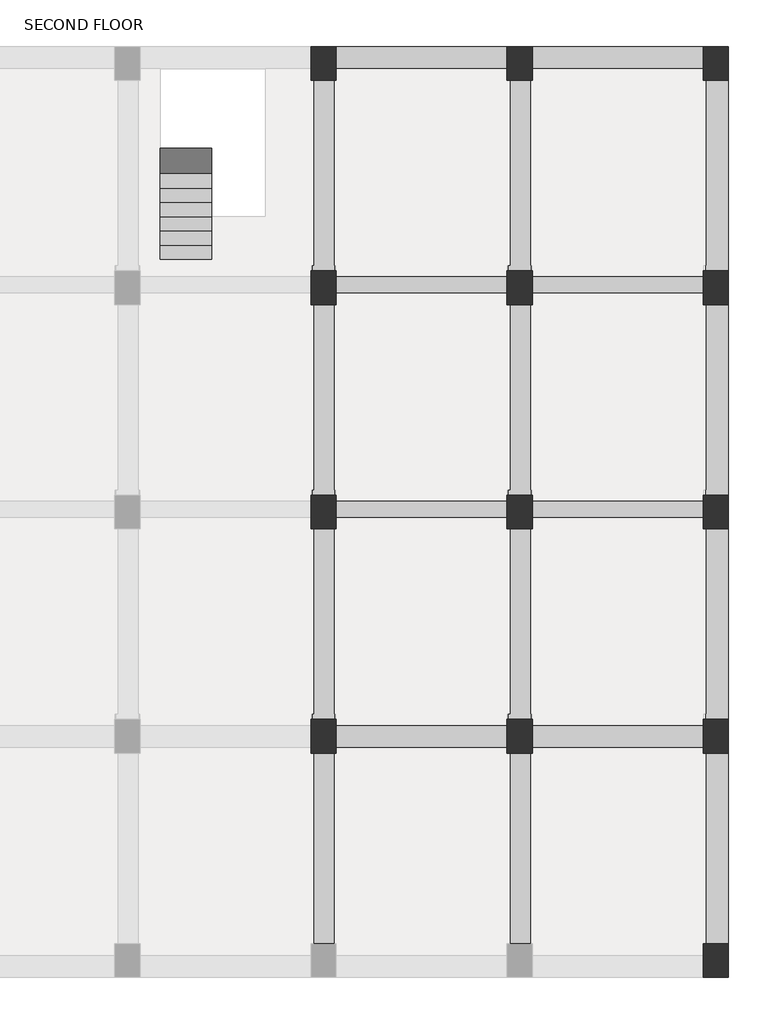
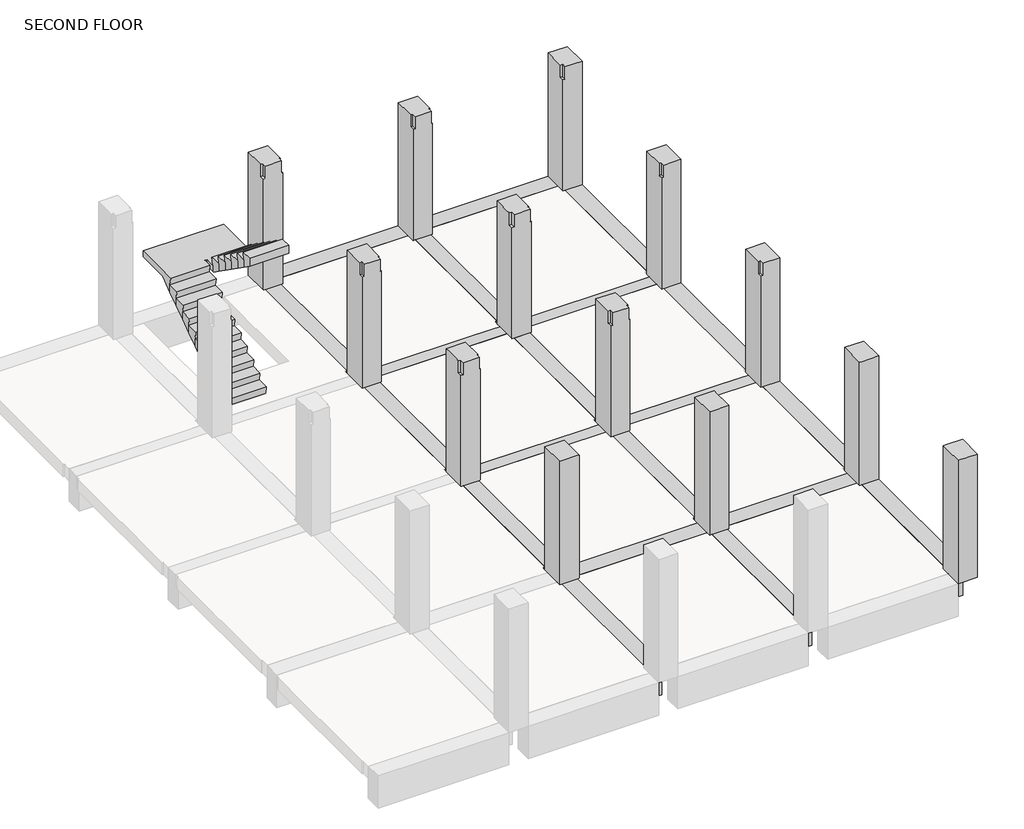
# One storey, part 3 of 3: 20 beams, 13 columns, 1 stair flight.
"""IFC4 building model written with IfcOpenShell, lengths in millimetres."""

from ifc_helpers import new_model, si_unit, origin, place, context, project, spatial, faceted_brep, element, save

model = new_model("IFC4")

# Units and contexts
model_context = context("Model", 3, world=origin())
ifc_project = project(units=[si_unit("LENGTHUNIT", "METRE", prefix="MILLI")], contexts=[model_context])

# Site, building, storey
site = spatial("IfcSite", under=ifc_project)
building = spatial("IfcBuilding", under=site)
storey = spatial("IfcBuildingStorey", under=building, Name="SECOND FLOOR", Elevation=6096.0)

# Beams
placement = place(None, origin())
element("IfcBeam", 1, ObjectType="M_Concrete-Rectangular Beam : 400 x 800mm", at=placement, inside=storey, context=model_context, shape_type="Brep", body=[
    faceted_brep([(7955.1115906, 15703.1212443, 6096.0), (8355.1115906, 15703.1212443, 6096.0), (8355.1115906, 19103.1212443, 6096.0), (7955.1115906, 19103.1212443, 6096.0), (7955.1115906, 15803.1212443, 6096.0), (7955.1115906, 15703.1212443, 5296.0), (7955.1115906, 19103.1212443, 5296.0), (8355.1115906, 15703.1212443, 5296.0), (8355.1115906, 19103.1212443, 5296.0)], [[[0, 1, 2, 3, 4]], [[5, 0, 4, 3, 6]], [[7, 5, 6, 8]], [[1, 7, 8, 2]], [[2, 8, 6, 3]], [[1, 0, 5, 7]]]),
])
element("IfcBeam", 2, ObjectType="M_Concrete-Rectangular Beam : 400 x 800mm", at=placement, inside=storey, context=model_context, shape_type="Brep", body=[
    faceted_brep([(7955.1115906, 11703.1212443, 6096.0), (8355.1115906, 11703.1212443, 6096.0), (8355.1115906, 15103.1212443, 6096.0), (7955.1115906, 15103.1212443, 6096.0), (7955.1115906, 11803.1212443, 6096.0), (7955.1115906, 11703.1212443, 5296.0), (7955.1115906, 15103.1212443, 5296.0), (8355.1115906, 11703.1212443, 5296.0), (8355.1115906, 15103.1212443, 5296.0)], [[[0, 1, 2, 3, 4]], [[5, 0, 4, 3, 6]], [[7, 5, 6, 8]], [[1, 7, 8, 2]], [[2, 8, 6, 3]], [[1, 0, 5, 7]]]),
])
element("IfcBeam", 3, ObjectType="M_Concrete-Rectangular Beam : 400 x 800mm", at=placement, inside=storey, context=model_context, shape_type="Brep", body=[
    faceted_brep([(7955.1115906, 7703.1212443, 6096.0), (8355.1115906, 7703.1212443, 6096.0), (8355.1115906, 11103.1212443, 6096.0), (7955.1115906, 11103.1212443, 6096.0), (7955.1115906, 7803.1212443, 6096.0), (7955.1115906, 7703.1212443, 5296.0), (7955.1115906, 11103.1212443, 5296.0), (8355.1115906, 7703.1212443, 5296.0), (8355.1115906, 11103.1212443, 5296.0)], [[[0, 1, 2, 3, 4]], [[5, 0, 4, 3, 6]], [[7, 5, 6, 8]], [[1, 7, 8, 2]], [[1, 0, 5, 7]], [[3, 2, 8, 6]]]),
])
element("IfcBeam", 4, ObjectType="M_Concrete-Rectangular Beam : 400 x 800mm", at=placement, inside=storey, context=model_context, shape_type="Brep", body=[
    faceted_brep([(8355.1115906, 7103.1212443, 6096.0), (7955.1115906, 7103.1212443, 6096.0), (7955.1115906, 3703.1212443, 6096.0), (8355.1115906, 3703.1212443, 6096.0), (7955.1115906, 7103.1212443, 5796.0), (7955.1115906, 7103.1212443, 5296.0), (7955.1115906, 3703.1212443, 5296.0), (7955.1115906, 3703.1212443, 5796.0), (8355.1115906, 7103.1212443, 5296.0), (8355.1115906, 3703.1212443, 5296.0)], [[[0, 1, 2, 3]], [[1, 4, 5, 6, 7, 2]], [[5, 8, 9, 6]], [[8, 0, 3, 9]], [[0, 8, 5, 4, 1]], [[3, 2, 7, 6, 9]]]),
])
element("IfcBeam", 5, ObjectType="M_Concrete-Rectangular Beam : 400 x 800mm", at=placement, inside=storey, context=model_context, shape_type="Brep", body=[
    faceted_brep([(1355.1115906, 19703.1212443, 6096.0), (1355.1115906, 19303.1212443, 6096.0), (4405.1115906, 19303.1212443, 6096.0), (4405.1115906, 19703.1212443, 6096.0), (1355.1115906, 19303.1212443, 5796.0), (1355.1115906, 19303.1212443, 5296.0), (4405.1115906, 19303.1212443, 5296.0), (4405.1115906, 19303.1212443, 5796.0), (1355.1115906, 19703.1212443, 5296.0), (4405.1115906, 19703.1212443, 5296.0)], [[[0, 1, 2, 3]], [[1, 4, 5, 6, 7, 2]], [[5, 8, 9, 6]], [[8, 0, 3, 9]], [[1, 0, 8, 5, 4]], [[3, 2, 7, 6, 9]]]),
])
element("IfcBeam", 6, ObjectType="M_Concrete-Rectangular Beam : 400 x 800mm", at=placement, inside=storey, context=model_context, shape_type="Brep", body=[
    faceted_brep([(4855.1115906, 19703.1212443, 6096.0), (4855.1115906, 19303.1212443, 6096.0), (7905.1115906, 19303.1212443, 6096.0), (7905.1115906, 19703.1212443, 6096.0), (4855.1115906, 19303.1212443, 5796.0), (4855.1115906, 19303.1212443, 5296.0), (7905.1115906, 19303.1212443, 5296.0), (7905.1115906, 19303.1212443, 5796.0), (4855.1115906, 19703.1212443, 5296.0), (7905.1115906, 19703.1212443, 5296.0)], [[[0, 1, 2, 3]], [[1, 4, 5, 6, 7, 2]], [[5, 8, 9, 6]], [[8, 0, 3, 9]], [[1, 0, 8, 5, 4]], [[3, 2, 7, 6, 9]]]),
])
element("IfcBeam", 7, ObjectType="M_Concrete-Rectangular Beam : 400 x 800mm", at=placement, inside=storey, context=model_context, shape_type="Brep", body=[
    faceted_brep([(1330.1115906, 15703.1212443, 6096.0), (1330.1115906, 15803.1212443, 6096.0), (1330.1115906, 19103.1212443, 6096.0), (955.1115906, 19103.1212443, 6096.0), (955.1115906, 15803.1212443, 6096.0), (930.1115906, 15803.1212443, 6096.0), (930.1115906, 15703.1212443, 6096.0), (930.1115906, 19103.1212443, 5296.0), (930.1115906, 15703.1212443, 5296.0), (930.1115906, 15803.1212443, 5796.0), (930.1115906, 19103.1212443, 5796.0), (1330.1115906, 19103.1212443, 5296.0), (1330.1115906, 15703.1212443, 5296.0), (955.1115906, 19103.1212443, 5796.0), (955.1115906, 15803.1212443, 5796.0)], [[[0, 1, 2, 3, 4, 5, 6]], [[7, 8, 6, 5, 9, 10]], [[7, 11, 12, 8]], [[11, 2, 1, 0, 12]], [[2, 11, 7, 10, 13, 3]], [[0, 6, 8, 12]], [[9, 14, 13, 10]], [[14, 4, 3, 13]], [[4, 14, 9, 5]]]),
])
element("IfcBeam", 8, ObjectType="M_Concrete-Rectangular Beam : 400 x 800mm", at=placement, inside=storey, context=model_context, shape_type="Brep", body=[
    faceted_brep([(1330.1115906, 11703.1212443, 6096.0), (1330.1115906, 11803.1212443, 6096.0), (1330.1115906, 15103.1212443, 6096.0), (955.1115906, 15103.1212443, 6096.0), (955.1115906, 11803.1212443, 6096.0), (930.1115906, 11803.1212443, 6096.0), (930.1115906, 11703.1212443, 6096.0), (930.1115906, 15103.1212443, 5296.0), (930.1115906, 11703.1212443, 5296.0), (930.1115906, 11803.1212443, 5796.0), (930.1115906, 15103.1212443, 5796.0), (1330.1115906, 15103.1212443, 5296.0), (1330.1115906, 11703.1212443, 5296.0), (955.1115906, 15103.1212443, 5796.0), (955.1115906, 11803.1212443, 5796.0)], [[[0, 1, 2, 3, 4, 5, 6]], [[7, 8, 6, 5, 9, 10]], [[8, 7, 11, 12]], [[2, 1, 0, 12, 11]], [[2, 11, 7, 10, 13, 3]], [[0, 6, 8, 12]], [[9, 14, 13, 10]], [[14, 4, 3, 13]], [[4, 14, 9, 5]]]),
])
element("IfcBeam", 9, ObjectType="M_Concrete-Rectangular Beam : 400 x 800mm", at=placement, inside=storey, context=model_context, shape_type="Brep", body=[
    faceted_brep([(1330.1115906, 7703.1212443, 6096.0), (1330.1115906, 7803.1212443, 6096.0), (1330.1115906, 11103.1212443, 6096.0), (955.1115906, 11103.1212443, 6096.0), (955.1115906, 7803.1212443, 6096.0), (930.1115906, 7803.1212443, 6096.0), (930.1115906, 7703.1212443, 6096.0), (930.1115906, 11103.1212443, 5296.0), (930.1115906, 7703.1212443, 5296.0), (930.1115906, 7803.1212443, 5796.0), (930.1115906, 11103.1212443, 5796.0), (1330.1115906, 11103.1212443, 5296.0), (1330.1115906, 7703.1212443, 5296.0), (955.1115906, 11103.1212443, 5796.0), (955.1115906, 7803.1212443, 5796.0)], [[[0, 1, 2, 3, 4, 5, 6]], [[7, 8, 6, 5, 9, 10]], [[7, 11, 12, 8]], [[11, 2, 1, 0, 12]], [[2, 11, 7, 10, 13, 3]], [[0, 6, 8, 12]], [[9, 14, 13, 10]], [[14, 4, 3, 13]], [[4, 14, 9, 5]]]),
])
element("IfcBeam", 10, ObjectType="M_Concrete-Rectangular Beam : 400 x 800mm", at=placement, inside=storey, context=model_context, shape_type="Brep", body=[
    faceted_brep([(1330.1115906, 3703.1212443, 6096.0), (1330.1115906, 7103.1212443, 6096.0), (955.1115906, 7103.1212443, 6096.0), (955.1115906, 3703.1212443, 6096.0), (930.1115906, 7103.1212443, 5296.0), (930.1115906, 3703.1212443, 5296.0), (930.1115906, 3703.1212443, 5796.0), (930.1115906, 7103.1212443, 5796.0), (1330.1115906, 7103.1212443, 5296.0), (1330.1115906, 3703.1212443, 5296.0), (1330.1115906, 7103.1212443, 5796.0), (1330.1115906, 3703.1212443, 5796.0), (955.1115906, 7103.1212443, 5796.0), (955.1115906, 3703.1212443, 5796.0)], [[[0, 1, 2, 3]], [[4, 5, 6, 7]], [[4, 8, 9, 5]], [[8, 10, 1, 0, 11, 9]], [[8, 4, 7, 12, 2, 1, 10]], [[5, 9, 11, 0, 3, 13, 6]], [[13, 12, 7, 6]], [[12, 13, 3, 2]]]),
])
element("IfcBeam", 11, ObjectType="M_Concrete-Rectangular Beam : 400 x 800mm", at=placement, inside=storey, context=model_context, shape_type="Brep", body=[
    faceted_brep([(4830.1115906, 15703.1212443, 6096.0), (4830.1115906, 15803.1212443, 6096.0), (4830.1115906, 19103.1212443, 6096.0), (4455.1115906, 19103.1212443, 6096.0), (4455.1115906, 15803.1212443, 6096.0), (4430.1115906, 15803.1212443, 6096.0), (4430.1115906, 15703.1212443, 6096.0), (4430.1115906, 19103.1212443, 5296.0), (4430.1115906, 15703.1212443, 5296.0), (4430.1115906, 15803.1212443, 5796.0), (4430.1115906, 19103.1212443, 5796.0), (4830.1115906, 19103.1212443, 5296.0), (4830.1115906, 15703.1212443, 5296.0), (4455.1115906, 19103.1212443, 5796.0), (4455.1115906, 15803.1212443, 5796.0)], [[[0, 1, 2, 3, 4, 5, 6]], [[7, 8, 6, 5, 9, 10]], [[8, 7, 11, 12]], [[2, 1, 0, 12, 11]], [[2, 11, 7, 10, 13, 3]], [[0, 6, 8, 12]], [[9, 14, 13, 10]], [[14, 4, 3, 13]], [[4, 14, 9, 5]]]),
])
element("IfcBeam", 12, ObjectType="M_Concrete-Rectangular Beam : 400 x 800mm", at=placement, inside=storey, context=model_context, shape_type="Brep", body=[
    faceted_brep([(4830.1115906, 11703.1212443, 6096.0), (4830.1115906, 11803.1212443, 6096.0), (4830.1115906, 15103.1212443, 6096.0), (4455.1115906, 15103.1212443, 6096.0), (4455.1115906, 11803.1212443, 6096.0), (4430.1115906, 11803.1212443, 6096.0), (4430.1115906, 11703.1212443, 6096.0), (4430.1115906, 15103.1212443, 5296.0), (4430.1115906, 11703.1212443, 5296.0), (4430.1115906, 11803.1212443, 5796.0), (4430.1115906, 15103.1212443, 5796.0), (4830.1115906, 15103.1212443, 5296.0), (4830.1115906, 11703.1212443, 5296.0), (4455.1115906, 15103.1212443, 5796.0), (4455.1115906, 11803.1212443, 5796.0)], [[[0, 1, 2, 3, 4, 5, 6]], [[7, 8, 6, 5, 9, 10]], [[7, 11, 12, 8]], [[11, 2, 1, 0, 12]], [[2, 11, 7, 10, 13, 3]], [[0, 6, 8, 12]], [[9, 14, 13, 10]], [[14, 4, 3, 13]], [[4, 14, 9, 5]]]),
])
element("IfcBeam", 13, ObjectType="M_Concrete-Rectangular Beam : 400 x 800mm", at=placement, inside=storey, context=model_context, shape_type="Brep", body=[
    faceted_brep([(4430.1115906, 7703.1212443, 6096.0), (4830.1115906, 7703.1212443, 6096.0), (4830.1115906, 7803.1212443, 6096.0), (4830.1115906, 11103.1212443, 6096.0), (4455.1115906, 11103.1212443, 6096.0), (4455.1115906, 7803.1212443, 6096.0), (4430.1115906, 7803.1212443, 6096.0), (4430.1115906, 7703.1212443, 5296.0), (4430.1115906, 7803.1212443, 5796.0), (4430.1115906, 11103.1212443, 5796.0), (4430.1115906, 11103.1212443, 5296.0), (4830.1115906, 7703.1212443, 5296.0), (4830.1115906, 11103.1212443, 5296.0), (4455.1115906, 11103.1212443, 5796.0), (4455.1115906, 7803.1212443, 5796.0)], [[[0, 1, 2, 3, 4, 5, 6]], [[7, 0, 6, 8, 9, 10]], [[11, 7, 10, 12]], [[1, 11, 12, 3, 2]], [[1, 0, 7, 11]], [[12, 10, 9, 13, 4, 3]], [[8, 14, 13, 9]], [[14, 5, 4, 13]], [[5, 14, 8, 6]]]),
])
element("IfcBeam", 14, ObjectType="M_Concrete-Rectangular Beam : 400 x 800mm", at=placement, inside=storey, context=model_context, shape_type="Brep", body=[
    faceted_brep([(4830.1115906, 3703.1212443, 6096.0), (4830.1115906, 7103.1212443, 6096.0), (4455.1115906, 7103.1212443, 6096.0), (4455.1115906, 3703.1212443, 6096.0), (4430.1115906, 7103.1212443, 5296.0), (4430.1115906, 3703.1212443, 5296.0), (4430.1115906, 3703.1212443, 5796.0), (4430.1115906, 7103.1212443, 5796.0), (4830.1115906, 7103.1212443, 5296.0), (4830.1115906, 3703.1212443, 5296.0), (4830.1115906, 7103.1212443, 5796.0), (4830.1115906, 3703.1212443, 5796.0), (4455.1115906, 7103.1212443, 5796.0), (4455.1115906, 3703.1212443, 5796.0)], [[[0, 1, 2, 3]], [[4, 5, 6, 7]], [[4, 8, 9, 5]], [[8, 10, 1, 0, 11, 9]], [[1, 10, 8, 4, 7, 12, 2]], [[5, 9, 11, 0, 3, 13, 6]], [[13, 12, 7, 6]], [[12, 13, 3, 2]]]),
])
element("IfcBeam", 15, ObjectType="M_Concrete-Rectangular Beam : 400 x 800mm", at=placement, inside=storey, context=model_context, shape_type="Brep", body=[
    faceted_brep([(4405.1115906, 15603.1212443, 6096.0), (1355.1115906, 15603.1212443, 6096.0), (1355.1115906, 15303.1212443, 6096.0), (4405.1115906, 15303.1212443, 6096.0), (1355.1115906, 15203.1212443, 5296.0), (4405.1115906, 15203.1212443, 5296.0), (4405.1115906, 15203.1212443, 5796.0), (1355.1115906, 15203.1212443, 5796.0), (1355.1115906, 15603.1212443, 5296.0), (4405.1115906, 15603.1212443, 5296.0), (1355.1115906, 15603.1212443, 5796.0), (4405.1115906, 15603.1212443, 5796.0), (1355.1115906, 15303.1212443, 5796.0), (4405.1115906, 15303.1212443, 5796.0)], [[[0, 1, 2, 3]], [[4, 5, 6, 7]], [[4, 8, 9, 5]], [[8, 10, 1, 0, 11, 9]], [[8, 4, 7, 12, 2, 1, 10]], [[5, 9, 11, 0, 3, 13, 6]], [[13, 12, 7, 6]], [[12, 13, 3, 2]]]),
])
element("IfcBeam", 16, ObjectType="M_Concrete-Rectangular Beam : 400 x 800mm", at=placement, inside=storey, context=model_context, shape_type="Brep", body=[
    faceted_brep([(7905.1115906, 15603.1212443, 6096.0), (4855.1115906, 15603.1212443, 6096.0), (4855.1115906, 15303.1212443, 6096.0), (7905.1115906, 15303.1212443, 6096.0), (4855.1115906, 15203.1212443, 5296.0), (7905.1115906, 15203.1212443, 5296.0), (7905.1115906, 15203.1212443, 5796.0), (4855.1115906, 15203.1212443, 5796.0), (4855.1115906, 15603.1212443, 5296.0), (7905.1115906, 15603.1212443, 5296.0), (4855.1115906, 15603.1212443, 5796.0), (7905.1115906, 15603.1212443, 5796.0), (4855.1115906, 15303.1212443, 5796.0), (7905.1115906, 15303.1212443, 5796.0)], [[[0, 1, 2, 3]], [[4, 5, 6, 7]], [[4, 8, 9, 5]], [[8, 10, 1, 0, 11, 9]], [[8, 4, 7, 12, 2, 1, 10]], [[5, 9, 11, 0, 3, 13, 6]], [[13, 12, 7, 6]], [[12, 13, 3, 2]]]),
])
element("IfcBeam", 17, ObjectType="M_Concrete-Rectangular Beam : 400 x 800mm", at=placement, inside=storey, context=model_context, shape_type="Brep", body=[
    faceted_brep([(7905.1115906, 11603.1212443, 6096.0), (4855.1115906, 11603.1212443, 6096.0), (4855.1115906, 11303.1212443, 6096.0), (7905.1115906, 11303.1212443, 6096.0), (4855.1115906, 11603.1212443, 5296.0), (4855.1115906, 11603.1212443, 5796.0), (7905.1115906, 11603.1212443, 5796.0), (7905.1115906, 11603.1212443, 5296.0), (4855.1115906, 11203.1212443, 5296.0), (7905.1115906, 11203.1212443, 5296.0), (7905.1115906, 11203.1212443, 5796.0), (4855.1115906, 11203.1212443, 5796.0), (4855.1115906, 11303.1212443, 5796.0), (7905.1115906, 11303.1212443, 5796.0)], [[[0, 1, 2, 3]], [[4, 5, 1, 0, 6, 7]], [[8, 4, 7, 9]], [[8, 9, 10, 11]], [[1, 5, 4, 8, 11, 12, 2]], [[7, 6, 0, 3, 13, 10, 9]], [[13, 12, 11, 10]], [[12, 13, 3, 2]]]),
])
element("IfcBeam", 18, ObjectType="M_Concrete-Rectangular Beam : 400 x 800mm", at=placement, inside=storey, context=model_context, shape_type="Brep", body=[
    faceted_brep([(4405.1115906, 11603.1212443, 6096.0), (1355.1115906, 11603.1212443, 6096.0), (1355.1115906, 11303.1212443, 6096.0), (4405.1115906, 11303.1212443, 6096.0), (1355.1115906, 11603.1212443, 5296.0), (1355.1115906, 11603.1212443, 5796.0), (4405.1115906, 11603.1212443, 5796.0), (4405.1115906, 11603.1212443, 5296.0), (1355.1115906, 11203.1212443, 5296.0), (4405.1115906, 11203.1212443, 5296.0), (4405.1115906, 11203.1212443, 5796.0), (1355.1115906, 11203.1212443, 5796.0), (1355.1115906, 11303.1212443, 5796.0), (4405.1115906, 11303.1212443, 5796.0)], [[[0, 1, 2, 3]], [[4, 5, 1, 0, 6, 7]], [[8, 4, 7, 9]], [[8, 9, 10, 11]], [[1, 5, 4, 8, 11, 12, 2]], [[7, 6, 0, 3, 13, 10, 9]], [[13, 12, 11, 10]], [[12, 13, 3, 2]]]),
])
element("IfcBeam", 19, ObjectType="M_Concrete-Rectangular Beam : 400 x 800mm", at=placement, inside=storey, context=model_context, shape_type="Brep", body=[
    faceted_brep([(1355.1115906, 7603.1212443, 6096.0), (1355.1115906, 7203.1212443, 6096.0), (4405.1115906, 7203.1212443, 6096.0), (4405.1115906, 7603.1212443, 6096.0), (1355.1115906, 7203.1212443, 5796.0), (1355.1115906, 7203.1212443, 5296.0), (4405.1115906, 7203.1212443, 5296.0), (4405.1115906, 7203.1212443, 5796.0), (1355.1115906, 7603.1212443, 5296.0), (4405.1115906, 7603.1212443, 5296.0), (1355.1115906, 7603.1212443, 5796.0), (4405.1115906, 7603.1212443, 5796.0)], [[[0, 1, 2, 3]], [[1, 4, 5, 6, 7, 2]], [[5, 8, 9, 6]], [[8, 10, 0, 3, 11, 9]], [[1, 0, 10, 8, 5, 4]], [[3, 2, 7, 6, 9, 11]]]),
])
element("IfcBeam", 20, ObjectType="M_Concrete-Rectangular Beam : 400 x 800mm", at=placement, inside=storey, context=model_context, shape_type="Brep", body=[
    faceted_brep([(4855.1115906, 7603.1212443, 6096.0), (4855.1115906, 7203.1212443, 6096.0), (7905.1115906, 7203.1212443, 6096.0), (7905.1115906, 7603.1212443, 6096.0), (4855.1115906, 7203.1212443, 5796.0), (4855.1115906, 7203.1212443, 5296.0), (7905.1115906, 7203.1212443, 5296.0), (7905.1115906, 7203.1212443, 5796.0), (4855.1115906, 7603.1212443, 5296.0), (7905.1115906, 7603.1212443, 5296.0), (4855.1115906, 7603.1212443, 5796.0), (7905.1115906, 7603.1212443, 5796.0)], [[[0, 1, 2, 3]], [[1, 4, 5, 6, 7, 2]], [[5, 8, 9, 6]], [[8, 10, 0, 3, 11, 9]], [[1, 0, 10, 8, 5, 4]], [[3, 2, 7, 6, 9, 11]]]),
])

# Columns
element("IfcColumn", 21, ObjectType="M_Concrete-Rectangular-Column : 450 x 600mm", at=placement, inside=storey, context=model_context, shape_type="Brep", body=[
    faceted_brep([(1355.1115906, 19703.1212443, 6096.0), (1355.1115906, 19103.1212443, 6096.0), (905.1115906, 19103.1212443, 6096.0), (905.1115906, 19703.1212443, 6096.0), (1355.1115906, 19703.1212443, 9144.0), (1355.1115906, 19303.1212443, 9144.0), (1355.1115906, 19203.1212443, 9144.0), (1355.1115906, 19203.1212443, 8844.0), (1355.1115906, 19103.1212443, 8844.0), (1330.1115906, 19103.1212443, 8844.0), (1330.1115906, 19103.1212443, 9144.0), (955.1115906, 19103.1212443, 9144.0), (955.1115906, 19103.1212443, 8844.0), (905.1115906, 19103.1212443, 8844.0), (905.1115906, 19203.1212443, 8844.0), (905.1115906, 19203.1212443, 9144.0), (905.1115906, 19303.1212443, 9144.0), (905.1115906, 19703.1212443, 9144.0), (955.1115906, 19203.1212443, 9144.0), (1330.1115906, 19203.1212443, 9144.0), (1330.1115906, 19203.1212443, 8844.0), (955.1115906, 19203.1212443, 8844.0)], [[[0, 1, 2, 3]], [[1, 0, 4, 5, 6, 7, 8]], [[2, 1, 8, 9, 10, 11, 12, 13]], [[3, 2, 13, 14, 15, 16, 17]], [[0, 3, 17, 4]], [[4, 17, 16, 15, 18, 11, 10, 19, 6, 5]], [[7, 20, 9, 8]], [[20, 19, 10, 9]], [[20, 7, 6, 19]], [[21, 14, 13, 12]], [[18, 21, 12, 11]], [[14, 21, 18, 15]]]),
])
element("IfcColumn", 22, ObjectType="M_Concrete-Rectangular-Column : 450 x 600mm", at=placement, inside=storey, context=model_context, shape_type="Brep", body=[
    faceted_brep([(4855.1115906, 19703.1212443, 6096.0), (4855.1115906, 19103.1212443, 6096.0), (4405.1115906, 19103.1212443, 6096.0), (4405.1115906, 19703.1212443, 6096.0), (4855.1115906, 19703.1212443, 9144.0), (4855.1115906, 19303.1212443, 9144.0), (4855.1115906, 19203.1212443, 9144.0), (4855.1115906, 19203.1212443, 8844.0), (4855.1115906, 19103.1212443, 8844.0), (4830.1115906, 19103.1212443, 8844.0), (4830.1115906, 19103.1212443, 9144.0), (4455.1115906, 19103.1212443, 9144.0), (4455.1115906, 19103.1212443, 8844.0), (4405.1115906, 19103.1212443, 8844.0), (4405.1115906, 19203.1212443, 8844.0), (4405.1115906, 19203.1212443, 9144.0), (4405.1115906, 19303.1212443, 9144.0), (4405.1115906, 19703.1212443, 9144.0), (4455.1115906, 19203.1212443, 9144.0), (4830.1115906, 19203.1212443, 9144.0), (4830.1115906, 19203.1212443, 8844.0), (4455.1115906, 19203.1212443, 8844.0)], [[[0, 1, 2, 3]], [[1, 0, 4, 5, 6, 7, 8]], [[2, 1, 8, 9, 10, 11, 12, 13]], [[3, 2, 13, 14, 15, 16, 17]], [[0, 3, 17, 4]], [[4, 17, 16, 15, 18, 11, 10, 19, 6, 5]], [[7, 20, 9, 8]], [[20, 19, 10, 9]], [[20, 7, 6, 19]], [[21, 14, 13, 12]], [[18, 21, 12, 11]], [[14, 21, 18, 15]]]),
])
element("IfcColumn", 23, ObjectType="M_Concrete-Rectangular-Column : 450 x 600mm", at=placement, inside=storey, context=model_context, shape_type="Brep", body=[
    faceted_brep([(8355.1115906, 19703.1212443, 6096.0), (8355.1115906, 19103.1212443, 6096.0), (7905.1115906, 19103.1212443, 6096.0), (7905.1115906, 19703.1212443, 6096.0), (8355.1115906, 19703.1212443, 9144.0), (8355.1115906, 19103.1212443, 9144.0), (7955.1115906, 19103.1212443, 9144.0), (7955.1115906, 19103.1212443, 8844.0), (7905.1115906, 19103.1212443, 8844.0), (7905.1115906, 19203.1212443, 8844.0), (7905.1115906, 19203.1212443, 9144.0), (7905.1115906, 19303.1212443, 9144.0), (7905.1115906, 19703.1212443, 9144.0), (7955.1115906, 19203.1212443, 9144.0), (7955.1115906, 19203.1212443, 8844.0)], [[[0, 1, 2, 3]], [[1, 0, 4, 5]], [[2, 1, 5, 6, 7, 8]], [[3, 2, 8, 9, 10, 11, 12]], [[0, 3, 12, 4]], [[5, 4, 12, 11, 10, 13, 6]], [[14, 9, 8, 7]], [[13, 14, 7, 6]], [[9, 14, 13, 10]]]),
])
element("IfcColumn", 24, ObjectType="M_Concrete-Rectangular-Column : 450 x 600mm", at=placement, inside=storey, context=model_context, shape_type="Brep", body=[
    faceted_brep([(1355.1115906, 15703.1212443, 6096.0), (1355.1115906, 15103.1212443, 6096.0), (905.1115906, 15103.1212443, 6096.0), (905.1115906, 15703.1212443, 6096.0), (1355.1115906, 15703.1212443, 8844.0), (1355.1115906, 15703.1212443, 9144.0), (1355.1115906, 15603.1212443, 9144.0), (1355.1115906, 15303.1212443, 9144.0), (1355.1115906, 15203.1212443, 9144.0), (1355.1115906, 15203.1212443, 8844.0), (1355.1115906, 15103.1212443, 8844.0), (1330.1115906, 15103.1212443, 8844.0), (1330.1115906, 15103.1212443, 9144.0), (955.1115906, 15103.1212443, 9144.0), (955.1115906, 15103.1212443, 8844.0), (905.1115906, 15103.1212443, 8844.0), (905.1115906, 15203.1212443, 8844.0), (905.1115906, 15203.1212443, 9144.0), (905.1115906, 15303.1212443, 9144.0), (905.1115906, 15603.1212443, 9144.0), (905.1115906, 15703.1212443, 9144.0), (905.1115906, 15703.1212443, 8844.0), (955.1115906, 15203.1212443, 9144.0), (1330.1115906, 15203.1212443, 9144.0), (1330.1115906, 15203.1212443, 8844.0), (955.1115906, 15203.1212443, 8844.0)], [[[0, 1, 2, 3]], [[1, 0, 4, 5, 6, 7, 8, 9, 10]], [[2, 1, 10, 11, 12, 13, 14, 15]], [[3, 2, 15, 16, 17, 18, 19, 20, 21]], [[0, 3, 21, 20, 5, 4]], [[5, 20, 19, 18, 17, 22, 13, 12, 23, 8, 7, 6]], [[9, 24, 11, 10]], [[24, 23, 12, 11]], [[24, 9, 8, 23]], [[25, 16, 15, 14]], [[22, 25, 14, 13]], [[16, 25, 22, 17]]]),
])
element("IfcColumn", 25, ObjectType="M_Concrete-Rectangular-Column : 450 x 600mm", at=placement, inside=storey, context=model_context, shape_type="Brep", body=[
    faceted_brep([(4855.1115906, 15703.1212443, 6096.0), (4855.1115906, 15103.1212443, 6096.0), (4405.1115906, 15103.1212443, 6096.0), (4405.1115906, 15703.1212443, 6096.0), (4855.1115906, 15703.1212443, 8844.0), (4855.1115906, 15703.1212443, 9144.0), (4855.1115906, 15603.1212443, 9144.0), (4855.1115906, 15303.1212443, 9144.0), (4855.1115906, 15203.1212443, 9144.0), (4855.1115906, 15203.1212443, 8844.0), (4855.1115906, 15103.1212443, 8844.0), (4830.1115906, 15103.1212443, 8844.0), (4830.1115906, 15103.1212443, 9144.0), (4455.1115906, 15103.1212443, 9144.0), (4455.1115906, 15103.1212443, 8844.0), (4405.1115906, 15103.1212443, 8844.0), (4405.1115906, 15203.1212443, 8844.0), (4405.1115906, 15203.1212443, 9144.0), (4405.1115906, 15303.1212443, 9144.0), (4405.1115906, 15603.1212443, 9144.0), (4405.1115906, 15703.1212443, 9144.0), (4405.1115906, 15703.1212443, 8844.0), (4455.1115906, 15203.1212443, 9144.0), (4830.1115906, 15203.1212443, 9144.0), (4830.1115906, 15203.1212443, 8844.0), (4455.1115906, 15203.1212443, 8844.0)], [[[0, 1, 2, 3]], [[1, 0, 4, 5, 6, 7, 8, 9, 10]], [[2, 1, 10, 11, 12, 13, 14, 15]], [[3, 2, 15, 16, 17, 18, 19, 20, 21]], [[0, 3, 21, 20, 5, 4]], [[5, 20, 19, 18, 17, 22, 13, 12, 23, 8, 7, 6]], [[9, 24, 11, 10]], [[24, 23, 12, 11]], [[24, 9, 8, 23]], [[25, 16, 15, 14]], [[22, 25, 14, 13]], [[16, 25, 22, 17]]]),
])
element("IfcColumn", 26, ObjectType="M_Concrete-Rectangular-Column : 450 x 600mm", at=placement, inside=storey, context=model_context, shape_type="Brep", body=[
    faceted_brep([(8355.1115906, 15703.1212443, 6096.0), (8355.1115906, 15103.1212443, 6096.0), (7905.1115906, 15103.1212443, 6096.0), (7905.1115906, 15703.1212443, 6096.0), (8355.1115906, 15703.1212443, 9144.0), (8355.1115906, 15103.1212443, 9144.0), (7955.1115906, 15103.1212443, 9144.0), (7955.1115906, 15103.1212443, 8844.0), (7905.1115906, 15103.1212443, 8844.0), (7905.1115906, 15203.1212443, 8844.0), (7905.1115906, 15203.1212443, 9144.0), (7905.1115906, 15303.1212443, 9144.0), (7905.1115906, 15603.1212443, 9144.0), (7905.1115906, 15703.1212443, 9144.0), (7905.1115906, 15703.1212443, 8844.0), (7955.1115906, 15203.1212443, 9144.0), (7955.1115906, 15203.1212443, 8844.0)], [[[0, 1, 2, 3]], [[1, 0, 4, 5]], [[2, 1, 5, 6, 7, 8]], [[3, 2, 8, 9, 10, 11, 12, 13, 14]], [[0, 3, 14, 13, 4]], [[5, 4, 13, 12, 11, 10, 15, 6]], [[16, 9, 8, 7]], [[15, 16, 7, 6]], [[9, 16, 15, 10]]]),
])
element("IfcColumn", 27, ObjectType="M_Concrete-Rectangular-Column : 450 x 600mm", at=placement, inside=storey, context=model_context, shape_type="Brep", body=[
    faceted_brep([(1355.1115906, 11703.1212443, 6096.0), (1355.1115906, 11103.1212443, 6096.0), (905.1115906, 11103.1212443, 6096.0), (905.1115906, 11703.1212443, 6096.0), (1355.1115906, 11703.1212443, 8844.0), (1355.1115906, 11703.1212443, 9144.0), (1355.1115906, 11603.1212443, 9144.0), (1355.1115906, 11303.1212443, 9144.0), (1355.1115906, 11203.1212443, 9144.0), (1355.1115906, 11203.1212443, 8844.0), (1355.1115906, 11103.1212443, 8844.0), (1330.1115906, 11103.1212443, 8844.0), (1330.1115906, 11103.1212443, 9144.0), (955.1115906, 11103.1212443, 9144.0), (955.1115906, 11103.1212443, 8844.0), (905.1115906, 11103.1212443, 8844.0), (905.1115906, 11203.1212443, 8844.0), (905.1115906, 11203.1212443, 9144.0), (905.1115906, 11303.1212443, 9144.0), (905.1115906, 11603.1212443, 9144.0), (905.1115906, 11703.1212443, 9144.0), (905.1115906, 11703.1212443, 8844.0), (955.1115906, 11203.1212443, 9144.0), (1330.1115906, 11203.1212443, 9144.0), (1330.1115906, 11203.1212443, 8844.0), (955.1115906, 11203.1212443, 8844.0)], [[[0, 1, 2, 3]], [[1, 0, 4, 5, 6, 7, 8, 9, 10]], [[2, 1, 10, 11, 12, 13, 14, 15]], [[3, 2, 15, 16, 17, 18, 19, 20, 21]], [[0, 3, 21, 20, 5, 4]], [[5, 20, 19, 18, 17, 22, 13, 12, 23, 8, 7, 6]], [[9, 24, 11, 10]], [[24, 23, 12, 11]], [[24, 9, 8, 23]], [[25, 16, 15, 14]], [[22, 25, 14, 13]], [[16, 25, 22, 17]]]),
])
element("IfcColumn", 28, ObjectType="M_Concrete-Rectangular-Column : 450 x 600mm", at=placement, inside=storey, context=model_context, shape_type="Brep", body=[
    faceted_brep([(4855.1115906, 11703.1212443, 6096.0), (4855.1115906, 11103.1212443, 6096.0), (4405.1115906, 11103.1212443, 6096.0), (4405.1115906, 11703.1212443, 6096.0), (4855.1115906, 11703.1212443, 8844.0), (4855.1115906, 11703.1212443, 9144.0), (4855.1115906, 11603.1212443, 9144.0), (4855.1115906, 11303.1212443, 9144.0), (4855.1115906, 11203.1212443, 9144.0), (4855.1115906, 11203.1212443, 8844.0), (4855.1115906, 11103.1212443, 8844.0), (4830.1115906, 11103.1212443, 8844.0), (4830.1115906, 11103.1212443, 9144.0), (4455.1115906, 11103.1212443, 9144.0), (4455.1115906, 11103.1212443, 8844.0), (4405.1115906, 11103.1212443, 8844.0), (4405.1115906, 11203.1212443, 8844.0), (4405.1115906, 11203.1212443, 9144.0), (4405.1115906, 11303.1212443, 9144.0), (4405.1115906, 11603.1212443, 9144.0), (4405.1115906, 11703.1212443, 9144.0), (4405.1115906, 11703.1212443, 8844.0), (4455.1115906, 11203.1212443, 9144.0), (4830.1115906, 11203.1212443, 9144.0), (4830.1115906, 11203.1212443, 8844.0), (4455.1115906, 11203.1212443, 8844.0)], [[[0, 1, 2, 3]], [[1, 0, 4, 5, 6, 7, 8, 9, 10]], [[2, 1, 10, 11, 12, 13, 14, 15]], [[3, 2, 15, 16, 17, 18, 19, 20, 21]], [[0, 3, 21, 20, 5, 4]], [[5, 20, 19, 18, 17, 22, 13, 12, 23, 8, 7, 6]], [[9, 24, 11, 10]], [[24, 23, 12, 11]], [[24, 9, 8, 23]], [[25, 16, 15, 14]], [[22, 25, 14, 13]], [[16, 25, 22, 17]]]),
])
element("IfcColumn", 29, ObjectType="M_Concrete-Rectangular-Column : 450 x 600mm", at=placement, inside=storey, context=model_context, shape_type="Brep", body=[
    faceted_brep([(8355.1115906, 11703.1212443, 6096.0), (8355.1115906, 11103.1212443, 6096.0), (7905.1115906, 11103.1212443, 6096.0), (7905.1115906, 11703.1212443, 6096.0), (8355.1115906, 11703.1212443, 9144.0), (8355.1115906, 11103.1212443, 9144.0), (7955.1115906, 11103.1212443, 9144.0), (7955.1115906, 11103.1212443, 8844.0), (7905.1115906, 11103.1212443, 8844.0), (7905.1115906, 11203.1212443, 8844.0), (7905.1115906, 11203.1212443, 9144.0), (7905.1115906, 11303.1212443, 9144.0), (7905.1115906, 11603.1212443, 9144.0), (7905.1115906, 11703.1212443, 9144.0), (7905.1115906, 11703.1212443, 8844.0), (7955.1115906, 11203.1212443, 9144.0), (7955.1115906, 11203.1212443, 8844.0)], [[[0, 1, 2, 3]], [[1, 0, 4, 5]], [[2, 1, 5, 6, 7, 8]], [[3, 2, 8, 9, 10, 11, 12, 13, 14]], [[0, 3, 14, 13, 4]], [[5, 4, 13, 12, 11, 10, 15, 6]], [[16, 9, 8, 7]], [[15, 16, 7, 6]], [[9, 16, 15, 10]]]),
])
element("IfcColumn", 30, ObjectType="M_Concrete-Rectangular-Column : 450 x 600mm", at=placement, inside=storey, context=model_context, shape_type="Brep", body=[
    faceted_brep([(1355.1115906, 7703.1212443, 6096.0), (1355.1115906, 7103.1212443, 6096.0), (905.1115906, 7103.1212443, 6096.0), (905.1115906, 7703.1212443, 6096.0), (1355.1115906, 7703.1212443, 8844.0), (1355.1115906, 7703.1212443, 9144.0), (1355.1115906, 7603.1212443, 9144.0), (1355.1115906, 7203.1212443, 9144.0), (1355.1115906, 7103.1212443, 9144.0), (1355.1115906, 7103.1212443, 8844.0), (1330.1115906, 7103.1212443, 9144.0), (955.1115906, 7103.1212443, 9144.0), (905.1115906, 7103.1212443, 9144.0), (905.1115906, 7103.1212443, 8844.0), (905.1115906, 7203.1212443, 9144.0), (905.1115906, 7603.1212443, 9144.0), (905.1115906, 7703.1212443, 9144.0), (905.1115906, 7703.1212443, 8844.0)], [[[0, 1, 2, 3]], [[1, 0, 4, 5, 6, 7, 8, 9]], [[2, 1, 9, 8, 10, 11, 12, 13]], [[3, 2, 13, 12, 14, 15, 16, 17]], [[0, 3, 17, 16, 5, 4]], [[5, 16, 15, 14, 12, 11, 10, 8, 7, 6]]]),
])
element("IfcColumn", 31, ObjectType="M_Concrete-Rectangular-Column : 450 x 600mm", at=placement, inside=storey, context=model_context, shape_type="Brep", body=[
    faceted_brep([(4855.1115906, 7703.1212443, 6096.0), (4855.1115906, 7103.1212443, 6096.0), (4405.1115906, 7103.1212443, 6096.0), (4405.1115906, 7703.1212443, 6096.0), (4855.1115906, 7703.1212443, 8844.0), (4855.1115906, 7703.1212443, 9144.0), (4855.1115906, 7603.1212443, 9144.0), (4855.1115906, 7203.1212443, 9144.0), (4855.1115906, 7103.1212443, 9144.0), (4855.1115906, 7103.1212443, 8844.0), (4830.1115906, 7103.1212443, 9144.0), (4455.1115906, 7103.1212443, 9144.0), (4405.1115906, 7103.1212443, 9144.0), (4405.1115906, 7103.1212443, 8844.0), (4405.1115906, 7203.1212443, 9144.0), (4405.1115906, 7603.1212443, 9144.0), (4405.1115906, 7703.1212443, 9144.0), (4405.1115906, 7703.1212443, 8844.0)], [[[0, 1, 2, 3]], [[1, 0, 4, 5, 6, 7, 8, 9]], [[2, 1, 9, 8, 10, 11, 12, 13]], [[3, 2, 13, 12, 14, 15, 16, 17]], [[0, 3, 17, 16, 5, 4]], [[5, 16, 15, 14, 12, 11, 10, 8, 7, 6]]]),
])
element("IfcColumn", 32, ObjectType="M_Concrete-Rectangular-Column : 450 x 600mm", at=placement, inside=storey, context=model_context, shape_type="Brep", body=[
    faceted_brep([(8355.1115906, 7703.1212443, 6096.0), (8355.1115906, 7103.1212443, 6096.0), (7905.1115906, 7103.1212443, 6096.0), (7905.1115906, 7703.1212443, 6096.0), (8355.1115906, 7703.1212443, 9144.0), (8355.1115906, 7103.1212443, 9144.0), (7955.1115906, 7103.1212443, 9144.0), (7905.1115906, 7103.1212443, 9144.0), (7905.1115906, 7103.1212443, 8844.0), (7905.1115906, 7203.1212443, 9144.0), (7905.1115906, 7603.1212443, 9144.0), (7905.1115906, 7703.1212443, 9144.0), (7905.1115906, 7703.1212443, 8844.0)], [[[0, 1, 2, 3]], [[1, 0, 4, 5]], [[2, 1, 5, 6, 7, 8]], [[3, 2, 8, 7, 9, 10, 11, 12]], [[0, 3, 12, 11, 4]], [[5, 4, 11, 10, 9, 7, 6]]]),
])
element("IfcColumn", 33, ObjectType="M_Concrete-Rectangular-Column : 450 x 600mm", at=placement, inside=storey, context=model_context, shape_type="Brep", body=[
    faceted_brep([(8355.1115906, 3703.1212443, 6096.0), (8355.1115906, 3103.1212443, 6096.0), (7905.1115906, 3103.1212443, 6096.0), (7905.1115906, 3703.1212443, 6096.0), (8355.1115906, 3703.1212443, 9144.0), (8355.1115906, 3103.1212443, 9144.0), (7905.1115906, 3103.1212443, 9144.0), (7905.1115906, 3503.1212443, 9144.0), (7905.1115906, 3703.1212443, 9144.0), (7905.1115906, 3703.1212443, 8844.0), (7955.1115906, 3703.1212443, 9144.0)], [[[0, 1, 2, 3]], [[1, 0, 4, 5]], [[2, 1, 5, 6]], [[3, 2, 6, 7, 8, 9]], [[0, 3, 9, 8, 10, 4]], [[5, 4, 10, 8, 7, 6]]]),
])

# Stair flight
element("IfcStairFlight", 34, ObjectType="25 mm Nosing", at=placement, inside=storey, context=model_context, shape_type="Brep", body=[
    faceted_brep([(-1784.8884094, 15908.7212443, 6275.2941176), (-870.4884094, 15908.7212443, 6275.2941176), (-870.4884094, 16187.7212443, 6275.2941176), (-1784.8884094, 16187.7212443, 6275.2941176), (-1784.8884094, 16187.7212443, 6096.0), (-1784.8884094, 15933.7212443, 6096.0), (-870.4884094, 15933.7212443, 6096.0), (-870.4884094, 16187.7212443, 6096.0), (-1784.8884094, 16162.7212443, 6454.5882353), (-870.4884094, 16162.7212443, 6454.5882353), (-870.4884094, 16441.7212443, 6454.5882353), (-1784.8884094, 16441.7212443, 6454.5882353), (-1784.8884094, 16441.7212443, 6270.9824819), (-1784.8884094, 16193.8293949, 6096.0), (-870.4884094, 16193.8293949, 6096.0), (-870.4884094, 16441.7212443, 6270.9824819), (-1784.8884094, 16416.7212443, 6633.8823529), (-870.4884094, 16416.7212443, 6633.8823529), (-870.4884094, 16695.7212443, 6633.8823529), (-1784.8884094, 16695.7212443, 6633.8823529), (-1784.8884094, 16695.7212443, 6450.2765996), (-870.4884094, 16695.7212443, 6450.2765996), (-1784.8884094, 16670.7212443, 6813.1764706), (-870.4884094, 16670.7212443, 6813.1764706), (-870.4884094, 16949.7212443, 6813.1764706), (-1784.8884094, 16949.7212443, 6813.1764706), (-1784.8884094, 16949.7212443, 6629.5707172), (-870.4884094, 16949.7212443, 6629.5707172), (-1784.8884094, 16924.7212443, 6992.4705882), (-870.4884094, 16924.7212443, 6992.4705882), (-870.4884094, 17203.7212443, 6992.4705882), (-1784.8884094, 17203.7212443, 6992.4705882), (-1784.8884094, 17203.7212443, 6808.8648349), (-870.4884094, 17203.7212443, 6808.8648349), (-1784.8884094, 17178.7212443, 7171.7647059), (-870.4884094, 17178.7212443, 7171.7647059), (-870.4884094, 17457.7212443, 7171.7647059), (-1784.8884094, 17457.7212443, 7171.7647059), (-1784.8884094, 17457.7212443, 6988.1589525), (-870.4884094, 17457.7212443, 6988.1589525), (-1784.8884094, 17432.7212443, 7351.0588235), (-870.4884094, 17432.7212443, 7351.0588235), (-870.4884094, 17711.7212443, 7351.0588235), (-1784.8884094, 17711.7212443, 7351.0588235), (-1784.8884094, 17711.7212443, 7167.4530702), (-870.4884094, 17711.7212443, 7167.4530702), (-1784.8884094, 17686.7212443, 7530.3529412), (-870.4884094, 17686.7212443, 7530.3529412), (-870.4884094, 17965.7212443, 7530.3529412), (-1784.8884094, 17965.7212443, 7530.3529412), (-1784.8884094, 17965.7212443, 7346.7471878), (-870.4884094, 17965.7212443, 7346.7471878), (-1784.8884094, 17940.7212443, 7709.6470588), (-870.4884094, 17940.7212443, 7709.6470588), (-870.4884094, 18219.7212443, 7709.6470588), (-1784.8884094, 18219.7212443, 7709.6470588), (-1784.8884094, 18219.7212443, 7526.0413055), (-870.4884094, 18219.7212443, 7526.0413055), (94.7115906, 18169.7212443, 7888.9411765), (94.7115906, 19303.1212443, 7888.9411765), (-1784.8884094, 19303.1212443, 7888.9411765), (-1784.8884094, 18521.3293949, 7888.9411765), (-1784.8884094, 18194.7212443, 7888.9411765), (-870.4884094, 18194.7212443, 7888.9411765), (-870.4884094, 18388.7212443, 7888.9411765), (-819.6884094, 18388.7212443, 7888.9411765), (-819.6884094, 18169.7212443, 7888.9411765), (94.7115906, 18169.7212443, 7738.9411765), (94.7115906, 19303.1212443, 7738.9411765), (-1784.8884094, 19303.1212443, 7738.9411765), (-1784.8884094, 18521.3293949, 7738.9411765), (-870.4884094, 18521.3293949, 7738.9411765), (-870.4884094, 18388.7212443, 7738.9411765), (-819.6884094, 18388.7212443, 7738.9411765), (-819.6884094, 18169.7212443, 7738.9411765), (94.7115906, 18194.7212443, 8068.2352941), (-819.6884094, 18194.7212443, 8068.2352941), (-819.6884094, 18122.1130937, 8068.2352941), (-819.6884094, 17915.7212443, 8068.2352941), (94.7115906, 17915.7212443, 8068.2352941), (94.7115906, 18122.1130937, 8068.2352941), (94.7115906, 17915.7212443, 7884.6295408), (94.7115906, 18122.1130937, 7738.9411765), (-819.6884094, 18122.1130937, 7738.9411765), (-819.6884094, 17915.7212443, 7884.6295408), (94.7115906, 17940.7212443, 8247.5294118), (-819.6884094, 17940.7212443, 8247.5294118), (-819.6884094, 17661.7212443, 8247.5294118), (94.7115906, 17661.7212443, 8247.5294118), (94.7115906, 17661.7212443, 8063.9236584), (-819.6884094, 17661.7212443, 8063.9236584), (94.7115906, 17686.7212443, 8426.8235294), (-819.6884094, 17686.7212443, 8426.8235294), (-819.6884094, 17407.7212443, 8426.8235294), (94.7115906, 17407.7212443, 8426.8235294), (94.7115906, 17407.7212443, 8243.2177761), (-819.6884094, 17407.7212443, 8243.2177761), (94.7115906, 17432.7212443, 8606.1176471), (-819.6884094, 17432.7212443, 8606.1176471), (-819.6884094, 17153.7212443, 8606.1176471), (94.7115906, 17153.7212443, 8606.1176471), (94.7115906, 17153.7212443, 8422.5118937), (-819.6884094, 17153.7212443, 8422.5118937), (94.7115906, 17178.7212443, 8785.4117647), (-819.6884094, 17178.7212443, 8785.4117647), (-819.6884094, 16899.7212443, 8785.4117647), (94.7115906, 16899.7212443, 8785.4117647), (94.7115906, 16899.7212443, 8601.8060114), (-819.6884094, 16899.7212443, 8601.8060114), (94.7115906, 16924.7212443, 8964.7058824), (-819.6884094, 16924.7212443, 8964.7058824), (-819.6884094, 16670.7212443, 8964.7058824), (94.7115906, 16670.7212443, 8964.7058824), (94.7115906, 16670.7212443, 8763.4530702), (-819.6884094, 16670.7212443, 8763.4530702)], [[[0, 1, 2, 3]], [[0, 3, 4, 5]], [[2, 1, 6, 7]], [[8, 9, 10, 11]], [[4, 3, 8, 11, 12, 13]], [[2, 7, 14, 15, 10, 9]], [[16, 17, 18, 19]], [[16, 19, 20, 12, 11]], [[18, 17, 10, 15, 21]], [[22, 23, 24, 25]], [[22, 25, 26, 20, 19]], [[24, 23, 18, 21, 27]], [[28, 29, 30, 31]], [[28, 31, 32, 26, 25]], [[30, 29, 24, 27, 33]], [[34, 35, 36, 37]], [[34, 37, 38, 32, 31]], [[36, 35, 30, 33, 39]], [[40, 41, 42, 43]], [[40, 43, 44, 38, 37]], [[42, 41, 36, 39, 45]], [[46, 47, 48, 49]], [[46, 49, 50, 44, 43]], [[48, 47, 42, 45, 51]], [[52, 53, 54, 55]], [[52, 55, 56, 50, 49]], [[54, 53, 48, 51, 57]], [[58, 59, 60, 61, 62, 63, 64, 65, 66]], [[59, 58, 67, 68]], [[60, 59, 68, 69]], [[55, 62, 61, 60, 69, 70, 56]], [[64, 63, 54, 57, 71, 72]], [[65, 64, 72, 73]], [[66, 65, 73, 74]], [[75, 76, 77, 78, 79, 80]], [[58, 75, 80, 79, 81, 82, 67]], [[76, 66, 74, 83, 84, 78, 77]], [[85, 86, 87, 88]], [[85, 88, 89, 81, 79]], [[87, 86, 78, 84, 90]], [[91, 92, 93, 94]], [[91, 94, 95, 89, 88]], [[93, 92, 87, 90, 96]], [[97, 98, 99, 100]], [[97, 100, 101, 95, 94]], [[99, 98, 93, 96, 102]], [[103, 104, 105, 106]], [[103, 106, 107, 101, 100]], [[105, 104, 99, 102, 108]], [[1, 0, 5, 6]], [[3, 2, 9, 8]], [[11, 10, 17, 16]], [[19, 18, 23, 22]], [[25, 24, 29, 28]], [[31, 30, 35, 34]], [[37, 36, 41, 40]], [[43, 42, 47, 46]], [[49, 48, 53, 52]], [[55, 54, 63, 62]], [[58, 66, 76, 75]], [[79, 78, 86, 85]], [[88, 87, 92, 91]], [[94, 93, 98, 97]], [[100, 99, 104, 103]], [[109, 110, 111, 112]], [[109, 112, 113, 107, 106]], [[111, 110, 105, 108, 114]], [[112, 111, 114, 113]], [[106, 105, 110, 109]], [[5, 4, 13, 14, 7, 6]], [[70, 71, 57, 51, 45, 39, 33, 27, 21, 15, 14, 13, 12, 20, 26, 32, 38, 44, 50, 56]], [[71, 70, 69, 68, 67, 82, 83, 74, 73, 72]], [[83, 82, 81, 89, 95, 101, 107, 113, 114, 108, 102, 96, 90, 84]]]),
])

save(model, "model.ifc")

# Revit data of these elements
# Type "M_Concrete-Rectangular Beam : 400 x 800mm"
#   Length [instance default] = 5' - 0"
#   b = 1' - 3.74803"
#   h = 2' - 7.49606"
#   Structural Material [instance default] = Concrete, Cast-in-Place gray
#   Assembly Code = ""
# Type "M_Concrete-Rectangular-Column : 450 x 600mm"
#   b = 1' - 5.71654"
#   h = 1' - 11.62205"
#   Structural Material [instance default] = Concrete, Cast-in-Place gray
# Elements 1, 2, 3, 4, 5, 6, 7, 8, 9, 10, 11, 12, 13, 14, 15, 16, 17, 18, 19, 20 (IfcBeam, "M_Concrete-Rectangular Beam : 400 x 800mm")
#   Structural Material = Concrete, Cast-in-Place gray
#   Phase Created = New Construction
#   Materials on its faces: "Concrete, Cast-in-Place gray"
# Elements 21, 22, 23, 24, 25, 26, 27, 28, 29, 30, 31, 32, 33 (IfcColumn, "M_Concrete-Rectangular-Column : 450 x 600mm")
#   Structural Material = Concrete, Cast-in-Place gray
#   Phase Created = New Construction
#   Materials on its faces: "Concrete, Cast-in-Place gray"
# Element 34 (IfcStairFlight, "25 mm Nosing")
#   Phase Created = New Construction
#   Materials on its faces: "Concrete, Cast In Situ"
# Materials
#   "Concrete, Cast-in-Place gray": class "Concrete", colour RGB 192 192 192, transparency 0, Description = "Cast-in-place concrete", Cost = 0
#   "Concrete, Cast In Situ": class "Concrete", colour RGB 192 192 192, transparency 0, Description = "physical material", Cost = 0
